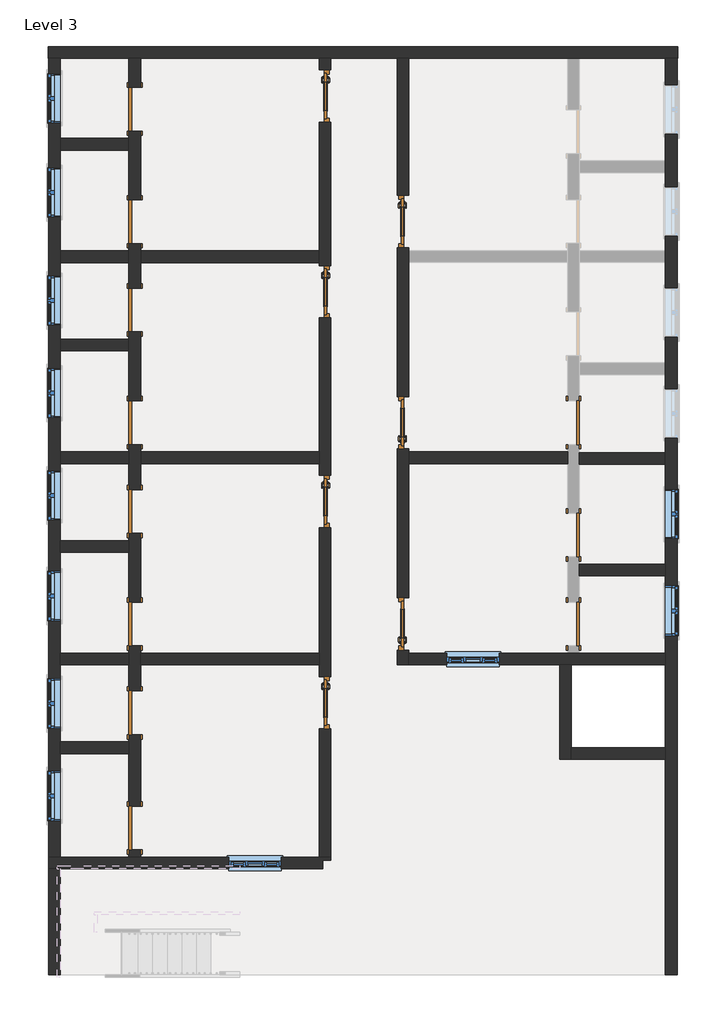
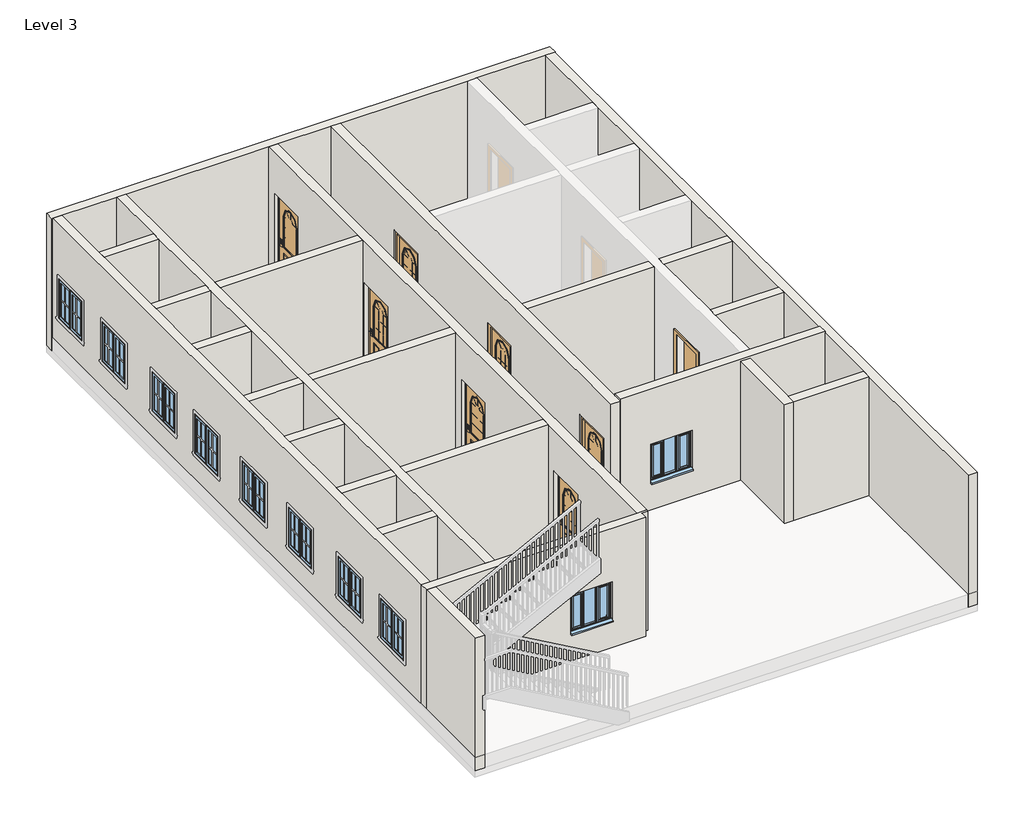
# One storey, part 1 of 4: 24 walls, 18 doors, 12 windows.
"""IFC4 building model written with IfcOpenShell, lengths in millimetres."""

from ifc_helpers import new_model, si_unit, frame, origin, place, context, project, spatial, polyline, outline, extrude, faceted_brep, transform, mapped, element, save
from components import doors_extsgl_w_glazing_bars_arched_910x2110mm_1ab485ba, doors_extsgl_w_glazing_bars_arched_910x2110mm_97dcda8a, door_fadea3f2, door_53b1b562, window_c29befe5, windows_tpl_plain_910x910mm_84e79c20

model = new_model("IFC4")

# Units and contexts
model_context = context("Model", 3, world=origin())
ifc_project = project(units=[si_unit("LENGTHUNIT", "METRE", prefix="MILLI")], contexts=[model_context])

# Site, building, storey
site = spatial("IfcSite", under=ifc_project)
building = spatial("IfcBuilding", under=site)
storey = spatial("IfcBuildingStorey", under=building, Name="Level 3", Elevation=6096.0)

# Doors
placement = place(None, origin())
doors_extsgl_w_glazing_bars_arched_910x2110mm_shape = doors_extsgl_w_glazing_bars_arched_910x2110mm_1ab485ba(model_context)
element("IfcDoor", 1, ObjectType="Doors_ExtSgl_w-Glazing_Bars_Arched : 910x2110mm", at=placement, inside=storey, context=model_context, shape_type="MappedRepresentation", body=[
    mapped(doors_extsgl_w_glazing_bars_arched_910x2110mm_shape, transform((-1635.1108866, 7135.2399728, 6096.0), x_axis=(0.0, -1.0, 0.0), y_axis=(1.0, 0.0, 0.0), z_axis=(0.0, 0.0, 1.0))),
])
element("IfcDoor", 2, ObjectType="Doors_ExtSgl_w-Glazing_Bars_Arched : 910x2110mm", at=placement, inside=storey, context=model_context, shape_type="MappedRepresentation", body=[
    mapped(doors_extsgl_w_glazing_bars_arched_910x2110mm_shape, transform((-1635.1108866, 3727.1935874, 6096.0), x_axis=(0.0, -1.0, 0.0), y_axis=(1.0, 0.0, 0.0), z_axis=(0.0, 0.0, 1.0))),
])
element("IfcDoor", 3, ObjectType="Doors_ExtSgl_w-Glazing_Bars_Arched : 910x2110mm", at=placement, inside=storey, context=model_context, shape_type="MappedRepresentation", body=[
    mapped(doors_extsgl_w_glazing_bars_arched_910x2110mm_shape, transform((-1635.1108866, 74.0399728, 6096.0), x_axis=(0.0, -1.0, 0.0), y_axis=(1.0, 0.0, 0.0), z_axis=(0.0, 0.0, 1.0))),
])
element("IfcDoor", 4, ObjectType="Doors_ExtSgl_w-Glazing_Bars_Arched : 910x2110mm", at=placement, inside=storey, context=model_context, shape_type="MappedRepresentation", body=[
    mapped(doors_extsgl_w_glazing_bars_arched_910x2110mm_shape, transform((-1635.1108866, -3431.1600272, 6096.0), x_axis=(0.0, -1.0, 0.0), y_axis=(1.0, 0.0, 0.0), z_axis=(0.0, 0.0, 1.0))),
])
element("IfcDoor", 5, ObjectType="Doors_ExtSgl_w-Glazing_Bars_Arched : 910x2110mm", at=placement, inside=storey, context=model_context, shape_type="MappedRepresentation", body=[
    mapped(doors_extsgl_w_glazing_bars_arched_910x2110mm_shape, transform((-276.2108866, -2059.5600272, 6096.0), x_axis=(0.0, 1.0, 0.0), y_axis=(-1.0, 0.0, 0.0), z_axis=(0.0, 0.0, 1.0))),
])
element("IfcDoor", 6, ObjectType="Doors_ExtSgl_w-Glazing_Bars_Arched : 910x2110mm", at=placement, inside=storey, context=model_context, shape_type="MappedRepresentation", body=[
    mapped(doors_extsgl_w_glazing_bars_arched_910x2110mm_shape, transform((-276.2108866, 1445.6399728, 6096.0), x_axis=(0.0, 1.0, 0.0), y_axis=(-1.0, 0.0, 0.0), z_axis=(0.0, 0.0, 1.0))),
])
doors_extsgl_w_glazing_bars_arched_910x2110mm_2_shape = doors_extsgl_w_glazing_bars_arched_910x2110mm_97dcda8a(model_context)
element("IfcDoor", 7, ObjectType="Doors_ExtSgl_w-Glazing_Bars_Arched : 910x2110mm", at=placement, inside=storey, context=model_context, shape_type="MappedRepresentation", body=[
    mapped(doors_extsgl_w_glazing_bars_arched_910x2110mm_2_shape, transform((-276.2108866, 4950.8399728, 6096.0), x_axis=(0.0, -1.0, 0.0), y_axis=(1.0, 0.0, 0.0), z_axis=(0.0, 0.0, 1.0))),
])
door_shape = door_fadea3f2(model_context)
element("IfcDoor", 8, ObjectType="Single-Flush : 30\" x 80\"", at=placement, inside=storey, context=model_context, shape_type="MappedRepresentation", body=[
    mapped(door_shape, transform((2695.5891134, -510.1600272, 6096.0), x_axis=(0.0, -1.0, 0.0), y_axis=(1.0, 0.0, 0.0), z_axis=(0.0, 0.0, 1.0))),
])
element("IfcDoor", 9, ObjectType="Single-Flush : 30\" x 80\"", at=placement, inside=storey, context=model_context, shape_type="MappedRepresentation", body=[
    mapped(door_shape, transform((2695.5891134, -2059.5600272, 6096.0), x_axis=(0.0, -1.0, 0.0), y_axis=(1.0, 0.0, 0.0), z_axis=(0.0, 0.0, 1.0))),
])
door_2_shape = door_53b1b562(model_context)
element("IfcDoor", 10, ObjectType="Single-Flush : 30\" x 80\"", at=placement, inside=storey, context=model_context, shape_type="MappedRepresentation", body=[
    mapped(door_2_shape, transform((-4949.8108866, 6906.6399728, 6096.0), x_axis=(0.0, -1.0, 0.0), y_axis=(1.0, 0.0, 0.0), z_axis=(0.0, 0.0, 1.0))),
])
element("IfcDoor", 11, ObjectType="Single-Flush : 30\" x 80\"", at=placement, inside=storey, context=model_context, shape_type="MappedRepresentation", body=[
    mapped(door_2_shape, transform((-4949.8108866, 4946.3935874, 6096.0), x_axis=(0.0, -1.0, 0.0), y_axis=(1.0, 0.0, 0.0), z_axis=(0.0, 0.0, 1.0))),
])
element("IfcDoor", 12, ObjectType="Single-Flush : 30\" x 80\"", at=placement, inside=storey, context=model_context, shape_type="MappedRepresentation", body=[
    mapped(door_2_shape, transform((-4949.8108866, 3407.538843, 6096.0), x_axis=(0.0, -1.0, 0.0), y_axis=(1.0, 0.0, 0.0), z_axis=(0.0, 0.0, 1.0))),
])
element("IfcDoor", 13, ObjectType="Single-Flush : 30\" x 80\"", at=placement, inside=storey, context=model_context, shape_type="MappedRepresentation", body=[
    mapped(door_2_shape, transform((-4949.8108866, 1445.6399728, 6096.0), x_axis=(0.0, -1.0, 0.0), y_axis=(1.0, 0.0, 0.0), z_axis=(0.0, 0.0, 1.0))),
])
element("IfcDoor", 14, ObjectType="Single-Flush : 30\" x 80\"", at=placement, inside=storey, context=model_context, shape_type="MappedRepresentation", body=[
    mapped(door_2_shape, transform((-4949.8108866, -103.7600272, 6096.0), x_axis=(0.0, -1.0, 0.0), y_axis=(1.0, 0.0, 0.0), z_axis=(0.0, 0.0, 1.0))),
])
element("IfcDoor", 15, ObjectType="Single-Flush : 30\" x 80\"", at=placement, inside=storey, context=model_context, shape_type="MappedRepresentation", body=[
    mapped(door_2_shape, transform((-4949.8108866, -2059.5600272, 6096.0), x_axis=(0.0, -1.0, 0.0), y_axis=(1.0, 0.0, 0.0), z_axis=(0.0, 0.0, 1.0))),
])
element("IfcDoor", 16, ObjectType="Single-Flush : 30\" x 80\"", at=placement, inside=storey, context=model_context, shape_type="MappedRepresentation", body=[
    mapped(door_2_shape, transform((-4949.8108866, -3608.9600272, 6096.0), x_axis=(0.0, -1.0, 0.0), y_axis=(1.0, 0.0, 0.0), z_axis=(0.0, 0.0, 1.0))),
])
element("IfcDoor", 17, ObjectType="Single-Flush : 30\" x 80\"", at=placement, inside=storey, context=model_context, shape_type="MappedRepresentation", body=[
    mapped(door_2_shape, transform((-4949.8108866, -5615.5600272, 6096.0), x_axis=(0.0, -1.0, 0.0), y_axis=(1.0, 0.0, 0.0), z_axis=(0.0, 0.0, 1.0))),
])
element("IfcDoor", 18, ObjectType="Single-Flush : 30\" x 80\"", at=placement, inside=storey, context=model_context, shape_type="MappedRepresentation", body=[
    mapped(door_2_shape, transform((2695.5891134, 1445.6399728, 6096.0), x_axis=(0.0, 1.0, 0.0), y_axis=(-1.0, 0.0, 0.0), z_axis=(0.0, 0.0, 1.0))),
])

# Walls
element("IfcWall", 19, ObjectType="4.5\" p", at=placement, inside=storey, context=model_context, shape_type="Brep", body=[
    faceted_brep([(-5051.4108866, -5996.5600272, 8128.0), (-5051.4108866, -5996.5600272, 6096.0), (-5051.4108866, -6123.5600272, 6096.0), (-5051.4108866, -6123.5600272, 9144.0), (-5051.4108866, -4320.1600272, 9144.0), (-5051.4108866, -4116.9600272, 9144.0), (-5051.4108866, -2770.7600272, 9144.0), (-5051.4108866, -2567.5600272, 9144.0), (-5051.4108866, -814.9600272, 9144.0), (-5051.4108866, -611.7600272, 9144.0), (-5051.4108866, 734.4399728, 9144.0), (-5051.4108866, 937.6399728, 9144.0), (-5051.4108866, 2696.338843, 9144.0), (-5051.4108866, 2899.538843, 9144.0), (-5051.4108866, 4235.1935874, 9144.0), (-5051.4108866, 4438.3935874, 9144.0), (-5051.4108866, 6195.4399728, 9144.0), (-5051.4108866, 6398.6399728, 9144.0), (-5051.4108866, 7795.6399728, 9144.0), (-5051.4108866, 7795.6399728, 6096.0), (-5051.4108866, 7287.6399728, 6096.0), (-5051.4108866, 7287.6399728, 8128.0), (-5051.4108866, 6525.6399728, 8128.0), (-5051.4108866, 6525.6399728, 6096.0), (-5051.4108866, 6398.6399728, 6096.0), (-5051.4108866, 6195.4399728, 6096.0), (-5051.4108866, 5327.3935874, 6096.0), (-5051.4108866, 5327.3935874, 8128.0), (-5051.4108866, 4565.3935874, 8128.0), (-5051.4108866, 4565.3935874, 6096.0), (-5051.4108866, 4438.3935874, 6096.0), (-5051.4108866, 4235.1935874, 6096.0), (-5051.4108866, 3788.538843, 6096.0), (-5051.4108866, 3788.538843, 8128.0), (-5051.4108866, 3026.538843, 8128.0), (-5051.4108866, 3026.538843, 6096.0), (-5051.4108866, 2899.538843, 6096.0), (-5051.4108866, 2696.338843, 6096.0), (-5051.4108866, 1826.6399728, 6096.0), (-5051.4108866, 1826.6399728, 8128.0), (-5051.4108866, 1064.6399728, 8128.0), (-5051.4108866, 1064.6399728, 6096.0), (-5051.4108866, 937.6399728, 6096.0), (-5051.4108866, 734.4399728, 6096.0), (-5051.4108866, 277.2399728, 6096.0), (-5051.4108866, 277.2399728, 8128.0), (-5051.4108866, -484.7600272, 8128.0), (-5051.4108866, -484.7600272, 6096.0), (-5051.4108866, -611.7600272, 6096.0), (-5051.4108866, -814.9600272, 6096.0), (-5051.4108866, -1678.5600272, 6096.0), (-5051.4108866, -1678.5600272, 8128.0), (-5051.4108866, -2440.5600272, 8128.0), (-5051.4108866, -2440.5600272, 6096.0), (-5051.4108866, -2567.5600272, 6096.0), (-5051.4108866, -2770.7600272, 6096.0), (-5051.4108866, -3227.9600272, 6096.0), (-5051.4108866, -3227.9600272, 8128.0), (-5051.4108866, -3989.9600272, 8128.0), (-5051.4108866, -3989.9600272, 6096.0), (-5051.4108866, -4116.9600272, 6096.0), (-5051.4108866, -4320.1600272, 6096.0), (-5051.4108866, -5234.5600272, 6096.0), (-5051.4108866, -5234.5600272, 8128.0), (-4848.2108866, -6123.5600272, 6096.0), (-4848.2108866, -5996.5600272, 6096.0), (-4848.2108866, -5996.5600272, 8128.0), (-4848.2108866, -5234.5600272, 8128.0), (-4848.2108866, -5234.5600272, 6096.0), (-4848.2108866, -3989.9600272, 6096.0), (-4848.2108866, -3989.9600272, 8128.0), (-4848.2108866, -3227.9600272, 8128.0), (-4848.2108866, -3227.9600272, 6096.0), (-4848.2108866, -2770.7600272, 6096.0), (-4848.2108866, -2567.5600272, 6096.0), (-4848.2108866, -2440.5600272, 6096.0), (-4848.2108866, -2440.5600272, 8128.0), (-4848.2108866, -1678.5600272, 8128.0), (-4848.2108866, -1678.5600272, 6096.0), (-4848.2108866, -484.7600272, 6096.0), (-4848.2108866, -484.7600272, 8128.0), (-4848.2108866, 277.2399728, 8128.0), (-4848.2108866, 277.2399728, 6096.0), (-4848.2108866, 734.4399728, 6096.0), (-4848.2108866, 937.6399728, 6096.0), (-4848.2108866, 1064.6399728, 6096.0), (-4848.2108866, 1064.6399728, 8128.0), (-4848.2108866, 1826.6399728, 8128.0), (-4848.2108866, 1826.6399728, 6096.0), (-4848.2108866, 3026.538843, 6096.0), (-4848.2108866, 3026.538843, 8128.0), (-4848.2108866, 3788.538843, 8128.0), (-4848.2108866, 3788.538843, 6096.0), (-4848.2108866, 4235.1935874, 6096.0), (-4848.2108866, 4438.3935874, 6096.0), (-4848.2108866, 4565.3935874, 6096.0), (-4848.2108866, 4565.3935874, 8128.0), (-4848.2108866, 5327.3935874, 8128.0), (-4848.2108866, 5327.3935874, 6096.0), (-4848.2108866, 6525.6399728, 6096.0), (-4848.2108866, 6525.6399728, 8128.0), (-4848.2108866, 7287.6399728, 8128.0), (-4848.2108866, 7287.6399728, 6096.0), (-4848.2108866, 7795.6399728, 6096.0), (-4848.2108866, 7795.6399728, 9144.0), (-4848.2108866, 4438.3935874, 9144.0), (-4848.2108866, 4235.1935874, 9144.0), (-4848.2108866, 937.6399728, 9144.0), (-4848.2108866, 734.4399728, 9144.0), (-4848.2108866, -2567.5600272, 9144.0), (-4848.2108866, -2770.7600272, 9144.0), (-4848.2108866, -6123.5600272, 9144.0)], [[[0, 1, 2, 3, 4, 5, 6, 7, 8, 9, 10, 11, 12, 13, 14, 15, 16, 17, 18, 19, 20, 21, 22, 23, 24, 25, 26, 27, 28, 29, 30, 31, 32, 33, 34, 35, 36, 37, 38, 39, 40, 41, 42, 43, 44, 45, 46, 47, 48, 49, 50, 51, 52, 53, 54, 55, 56, 57, 58, 59, 60, 61, 62, 63]], [[64, 65, 66, 67, 68, 69, 70, 71, 72, 73, 74, 75, 76, 77, 78, 79, 80, 81, 82, 83, 84, 85, 86, 87, 88, 89, 90, 91, 92, 93, 94, 95, 96, 97, 98, 99, 100, 101, 102, 103, 104, 105, 106, 107, 108, 109, 110, 111]], [[20, 19, 103, 102]], [[26, 25, 24, 23, 99, 98]], [[32, 31, 30, 29, 95, 94, 93, 92]], [[38, 37, 36, 35, 89, 88]], [[44, 43, 42, 41, 85, 84, 83, 82]], [[50, 49, 48, 47, 79, 78]], [[56, 55, 54, 53, 75, 74, 73, 72]], [[2, 1, 65, 64]], [[62, 61, 60, 59, 69, 68]], [[18, 17, 16, 15, 14, 13, 12, 11, 10, 9, 8, 7, 6, 5, 4, 3, 111, 110, 109, 108, 107, 106, 105, 104]], [[19, 18, 104, 103]], [[3, 2, 64, 111]], [[100, 99, 23, 22]], [[101, 100, 22, 21]], [[102, 101, 21, 20]], [[96, 95, 29, 28]], [[97, 96, 28, 27]], [[98, 97, 27, 26]], [[90, 89, 35, 34]], [[91, 90, 34, 33]], [[92, 91, 33, 32]], [[86, 85, 41, 40]], [[87, 86, 40, 39]], [[88, 87, 39, 38]], [[80, 79, 47, 46]], [[81, 80, 46, 45]], [[82, 81, 45, 44]], [[76, 75, 53, 52]], [[77, 76, 52, 51]], [[78, 77, 51, 50]], [[70, 69, 59, 58]], [[71, 70, 58, 57]], [[72, 71, 57, 56]], [[66, 65, 1, 0]], [[67, 66, 0, 63]], [[68, 67, 63, 62]]]),
])
element("IfcWall", 20, ObjectType="4.5\" p", at=placement, inside=storey, context=model_context, shape_type="SweptSolid", body=[
    extrude(outline(polyline([(-5051.4108866, 6195.4399728), (-6245.2108866, 6195.4399728), (-6245.2108866, 6398.6399728), (-5051.4108866, 6398.6399728), (-5051.4108866, 6195.4399728)])), frame((0.0, 0.0, 6096.0), z_axis=(0.0, 0.0, 1.0), x_axis=(1.0, 0.0, 0.0)), (0.0, 0.0, 1.0), 3048.0),
])
element("IfcWall", 21, ObjectType="4.5\" p", at=placement, inside=storey, context=model_context, shape_type="SweptSolid", body=[
    extrude(outline(polyline([(-5051.4108866, 4235.1935874), (-6245.2108866, 4235.1935874), (-6245.2108866, 4438.3935874), (-5051.4108866, 4438.3935874), (-5051.4108866, 4235.1935874)])), frame((0.0, 0.0, 6096.0), z_axis=(0.0, 0.0, 1.0), x_axis=(1.0, 0.0, 0.0)), (0.0, 0.0, 1.0), 3048.0),
])
element("IfcWall", 22, ObjectType="4.5\" p", at=placement, inside=storey, context=model_context, shape_type="SweptSolid", body=[
    extrude(outline(polyline([(-5051.4108866, 2696.338843), (-6245.2108866, 2696.338843), (-6245.2108866, 2899.538843), (-5051.4108866, 2899.538843), (-5051.4108866, 2696.338843)])), frame((0.0, 0.0, 6096.0), z_axis=(0.0, 0.0, 1.0), x_axis=(1.0, 0.0, 0.0)), (0.0, 0.0, 1.0), 3048.0),
])
element("IfcWall", 23, ObjectType="4.5\" p", at=placement, inside=storey, context=model_context, shape_type="SweptSolid", body=[
    extrude(outline(polyline([(-5051.4108866, 734.4399728), (-6245.2108866, 734.4399728), (-6245.2108866, 937.6399728), (-5051.4108866, 937.6399728), (-5051.4108866, 734.4399728)])), frame((0.0, 0.0, 6096.0), z_axis=(0.0, 0.0, 1.0), x_axis=(1.0, 0.0, 0.0)), (0.0, 0.0, 1.0), 3048.0),
])
element("IfcWall", 24, ObjectType="4.5\" p", at=placement, inside=storey, context=model_context, shape_type="SweptSolid", body=[
    extrude(outline(polyline([(-5051.4108866, -814.9600272), (-6245.2108866, -814.9600272), (-6245.2108866, -611.7600272), (-5051.4108866, -611.7600272), (-5051.4108866, -814.9600272)])), frame((0.0, 0.0, 6096.0), z_axis=(0.0, 0.0, 1.0), x_axis=(1.0, 0.0, 0.0)), (0.0, 0.0, 1.0), 3048.0),
])
element("IfcWall", 25, ObjectType="4.5\" p", at=placement, inside=storey, context=model_context, shape_type="SweptSolid", body=[
    extrude(outline(polyline([(-5051.4108866, -2770.7600272), (-6245.2108866, -2770.7600272), (-6245.2108866, -2567.5600272), (-5051.4108866, -2567.5600272), (-5051.4108866, -2770.7600272)])), frame((0.0, 0.0, 6096.0), z_axis=(0.0, 0.0, 1.0), x_axis=(1.0, 0.0, 0.0)), (0.0, 0.0, 1.0), 3048.0),
])
element("IfcWall", 26, ObjectType="4.5\" p", at=placement, inside=storey, context=model_context, shape_type="SweptSolid", body=[
    extrude(outline(polyline([(-5051.4108866, -4320.1600272), (-6245.2108866, -4320.1600272), (-6245.2108866, -4116.9600272), (-5051.4108866, -4116.9600272), (-5051.4108866, -4320.1600272)])), frame((0.0, 0.0, 6096.0), z_axis=(0.0, 0.0, 1.0), x_axis=(1.0, 0.0, 0.0)), (0.0, 0.0, 1.0), 3048.0),
])
element("IfcWall", 27, ObjectType="4.5\" p", at=placement, inside=storey, context=model_context, shape_type="Brep", body=[
    faceted_brep([(-1736.7108866, -3886.1600272, 8206.0), (-1736.7108866, -3886.1600272, 6096.0), (-1736.7108866, -6123.5600272, 6096.0), (-1736.7108866, -6123.5600272, 9144.0), (-1736.7108866, -2770.7600272, 9144.0), (-1736.7108866, -2567.5600272, 9144.0), (-1736.7108866, 734.4399728, 9144.0), (-1736.7108866, 937.6399728, 9144.0), (-1736.7108866, 4235.1935874, 9144.0), (-1736.7108866, 4438.3935874, 9144.0), (-1736.7108866, 7795.6399728, 9144.0), (-1736.7108866, 7795.6399728, 6096.0), (-1736.7108866, 7590.2399728, 6096.0), (-1736.7108866, 7590.2399728, 8206.0), (-1736.7108866, 6680.2399728, 8206.0), (-1736.7108866, 6680.2399728, 6096.0), (-1736.7108866, 4438.3935874, 6096.0), (-1736.7108866, 4235.1935874, 6096.0), (-1736.7108866, 4182.1935874, 6096.0), (-1736.7108866, 4182.1935874, 8206.0), (-1736.7108866, 3272.1935874, 8206.0), (-1736.7108866, 3272.1935874, 6096.0), (-1736.7108866, 937.6399728, 6096.0), (-1736.7108866, 734.4399728, 6096.0), (-1736.7108866, 529.0399728, 6096.0), (-1736.7108866, 529.0399728, 8206.0), (-1736.7108866, -380.9600272, 8206.0), (-1736.7108866, -380.9600272, 6096.0), (-1736.7108866, -2567.5600272, 6096.0), (-1736.7108866, -2770.7600272, 6096.0), (-1736.7108866, -2976.1600272, 6096.0), (-1736.7108866, -2976.1600272, 8206.0), (-1533.5108866, -6123.5600272, 6096.0), (-1533.5108866, -3886.1600272, 6096.0), (-1533.5108866, -3886.1600272, 8206.0), (-1533.5108866, -2976.1600272, 8206.0), (-1533.5108866, -2976.1600272, 6096.0), (-1533.5108866, -380.9600272, 6096.0), (-1533.5108866, -380.9600272, 8206.0), (-1533.5108866, 529.0399728, 8206.0), (-1533.5108866, 529.0399728, 6096.0), (-1533.5108866, 3272.1935874, 6096.0), (-1533.5108866, 3272.1935874, 8206.0), (-1533.5108866, 4182.1935874, 8206.0), (-1533.5108866, 4182.1935874, 6096.0), (-1533.5108866, 6680.2399728, 6096.0), (-1533.5108866, 6680.2399728, 8206.0), (-1533.5108866, 7590.2399728, 8206.0), (-1533.5108866, 7590.2399728, 6096.0), (-1533.5108866, 7795.6399728, 6096.0), (-1533.5108866, 7795.6399728, 9144.0), (-1533.5108866, -6123.5600272, 9144.0)], [[[0, 1, 2, 3, 4, 5, 6, 7, 8, 9, 10, 11, 12, 13, 14, 15, 16, 17, 18, 19, 20, 21, 22, 23, 24, 25, 26, 27, 28, 29, 30, 31]], [[32, 33, 34, 35, 36, 37, 38, 39, 40, 41, 42, 43, 44, 45, 46, 47, 48, 49, 50, 51]], [[12, 11, 49, 48]], [[18, 17, 16, 15, 45, 44]], [[24, 23, 22, 21, 41, 40]], [[2, 1, 33, 32]], [[30, 29, 28, 27, 37, 36]], [[10, 9, 8, 7, 6, 5, 4, 3, 51, 50]], [[3, 2, 32, 51]], [[11, 10, 50, 49]], [[48, 47, 13, 12]], [[46, 45, 15, 14]], [[47, 46, 14, 13]], [[44, 43, 19, 18]], [[42, 41, 21, 20]], [[43, 42, 20, 19]], [[40, 39, 25, 24]], [[38, 37, 27, 26]], [[39, 38, 26, 25]], [[36, 35, 31, 30]], [[34, 33, 1, 0]], [[35, 34, 0, 31]]]),
])
element("IfcWall", 28, ObjectType="4.5\" p", at=placement, inside=storey, context=model_context, shape_type="SweptSolid", body=[
    extrude(outline(polyline([(-1736.7108866, 4235.1935874), (-4848.2108866, 4235.1935874), (-4848.2108866, 4438.3935874), (-1736.7108866, 4438.3935874), (-1736.7108866, 4235.1935874)])), frame((0.0, 0.0, 6096.0), z_axis=(0.0, 0.0, 1.0), x_axis=(1.0, 0.0, 0.0)), (0.0, 0.0, 1.0), 3048.0),
])
element("IfcWall", 29, ObjectType="4.5\" p", at=placement, inside=storey, context=model_context, shape_type="SweptSolid", body=[
    extrude(outline(polyline([(-1736.7108866, 734.4399728), (-4848.2108866, 734.4399728), (-4848.2108866, 937.6399728), (-1736.7108866, 937.6399728), (-1736.7108866, 734.4399728)])), frame((0.0, 0.0, 6096.0), z_axis=(0.0, 0.0, 1.0), x_axis=(1.0, 0.0, 0.0)), (0.0, 0.0, 1.0), 3048.0),
])
element("IfcWall", 30, ObjectType="4.5\" p", at=placement, inside=storey, context=model_context, shape_type="SweptSolid", body=[
    extrude(outline(polyline([(-1736.7108866, -2770.7600272), (-4848.2108866, -2770.7600272), (-4848.2108866, -2567.5600272), (-1736.7108866, -2567.5600272), (-1736.7108866, -2770.7600272)])), frame((0.0, 0.0, 6096.0), z_axis=(0.0, 0.0, 1.0), x_axis=(1.0, 0.0, 0.0)), (0.0, 0.0, 1.0), 3048.0),
])
element("IfcWall", 31, ObjectType="4.5\" p", at=placement, inside=storey, context=model_context, shape_type="Brep", body=[
    faceted_brep([(-377.8108866, 4495.8399728, 8206.0), (-377.8108866, 4495.8399728, 6096.0), (-377.8108866, 1900.6399728, 6096.0), (-377.8108866, 1900.6399728, 8206.0), (-377.8108866, 990.6399728, 8206.0), (-377.8108866, 990.6399728, 6096.0), (-377.8108866, -1604.5600272, 6096.0), (-377.8108866, -1604.5600272, 8206.0), (-377.8108866, -2514.5600272, 8206.0), (-377.8108866, -2514.5600272, 6096.0), (-377.8108866, -2770.7600272, 6096.0), (-377.8108866, -2770.7600272, 9144.0), (-377.8108866, 7795.6399728, 9144.0), (-377.8108866, 7795.6399728, 6096.0), (-377.8108866, 5405.8399728, 6096.0), (-377.8108866, 5405.8399728, 8206.0), (-174.6108866, 1900.6399728, 6096.0), (-174.6108866, 4239.6399728, 6096.0), (-174.6108866, 4442.8399728, 6096.0), (-174.6108866, 4495.8399728, 6096.0), (-174.6108866, 4495.8399728, 8206.0), (-174.6108866, 5405.8399728, 8206.0), (-174.6108866, 5405.8399728, 6096.0), (-174.6108866, 7795.6399728, 6096.0), (-174.6108866, 7795.6399728, 9144.0), (-174.6108866, 4442.8399728, 9144.0), (-174.6108866, 4239.6399728, 9144.0), (-174.6108866, 937.6399728, 9144.0), (-174.6108866, 734.4399728, 9144.0), (-174.6108866, -2770.7600272, 9144.0), (-174.6108866, -2770.7600272, 6096.0), (-174.6108866, -2567.5600272, 6096.0), (-174.6108866, -2514.5600272, 6096.0), (-174.6108866, -2514.5600272, 8206.0), (-174.6108866, -1604.5600272, 8206.0), (-174.6108866, -1604.5600272, 6096.0), (-174.6108866, 734.4399728, 6096.0), (-174.6108866, 937.6399728, 6096.0), (-174.6108866, 990.6399728, 6096.0), (-174.6108866, 990.6399728, 8206.0), (-174.6108866, 1900.6399728, 8206.0)], [[[0, 1, 2, 3, 4, 5, 6, 7, 8, 9, 10, 11, 12, 13, 14, 15]], [[16, 17, 18, 19, 20, 21, 22, 23, 24, 25, 26, 27, 28, 29, 30, 31, 32, 33, 34, 35, 36, 37, 38, 39, 40]], [[32, 31, 30, 10, 9]], [[38, 37, 36, 35, 6, 5]], [[14, 13, 23, 22]], [[2, 1, 19, 18, 17, 16]], [[12, 11, 29, 28, 27, 26, 25, 24]], [[13, 12, 24, 23]], [[11, 10, 30, 29]], [[9, 8, 33, 32]], [[7, 6, 35, 34]], [[8, 7, 34, 33]], [[5, 4, 39, 38]], [[3, 2, 16, 40]], [[4, 3, 40, 39]], [[22, 21, 15, 14]], [[20, 19, 1, 0]], [[21, 20, 0, 15]]]),
])
element("IfcWall", 32, ObjectType="4.5\" p", at=placement, inside=storey, context=model_context, shape_type="Brep", body=[
    faceted_brep([(-174.6108866, -2770.7600272, 6096.0), (2454.2891134, -2770.7600272, 6096.0), (2657.4891134, -2770.7600272, 6096.0), (4295.7891134, -2770.7600272, 6096.0), (4295.7891134, -2770.7600272, 9184.1226014), (-174.6108866, -2770.7600272, 9184.1226014), (-174.6108866, -2770.7600272, 9144.0), (1397.9891134, -2770.7600272, 7920.4), (1397.9891134, -2770.7600272, 7010.4), (487.9891134, -2770.7600272, 7010.4), (487.9891134, -2770.7600272, 7920.4), (-174.6108866, -2567.5600272, 6096.0), (-174.6108866, -2567.5600272, 9184.1226014), (4295.7891134, -2567.5600272, 9184.1226014), (4295.7891134, -2567.5600272, 6096.0), (2797.1891134, -2567.5600272, 6096.0), (2593.9891134, -2567.5600272, 6096.0), (1397.9891134, -2567.5600272, 7920.4), (487.9891134, -2567.5600272, 7920.4), (487.9891134, -2567.5600272, 7010.4), (1397.9891134, -2567.5600272, 7010.4)], [[[0, 1, 2, 3, 4, 5, 6], [7, 8, 9, 10]], [[11, 12, 13, 14, 15, 16], [17, 18, 19, 20]], [[3, 2, 1, 0, 11, 16, 15, 14]], [[5, 4, 13, 12]], [[0, 6, 5, 12, 11]], [[4, 3, 14, 13]], [[8, 7, 17, 20]], [[9, 8, 20, 19]], [[10, 9, 19, 18]], [[7, 10, 18, 17]]]),
])
element("IfcWall", 33, ObjectType="4.5\" p", at=placement, inside=storey, context=model_context, shape_type="Brep", body=[
    faceted_brep([(2454.2891134, -2770.7600272, 6096.0), (2454.2891134, -4421.7600272, 6096.0), (2454.2891134, -4421.7600272, 9144.0), (2454.2891134, -2770.7600272, 9144.0), (2657.4891134, -2770.7600272, 6096.0), (2657.4891134, -2770.7600272, 9144.0), (2657.4891134, -4218.5600272, 9144.0), (2657.4891134, -4421.7600272, 9144.0), (2657.4891134, -4421.7600272, 6096.0), (2657.4891134, -4218.5600272, 6096.0)], [[[0, 1, 2, 3]], [[4, 5, 6, 7, 8, 9]], [[1, 0, 4, 9, 8]], [[3, 2, 7, 6, 5]], [[0, 3, 5, 4]], [[2, 1, 8, 7]]]),
])
element("IfcWall", 34, ObjectType="4.5\" p", at=placement, inside=storey, context=model_context, shape_type="SweptSolid", body=[
    extrude(outline(polyline([(2657.4891134, -4218.5600272), (4295.7891134, -4218.5600272), (4295.7891134, -4421.7600272), (2657.4891134, -4421.7600272), (2657.4891134, -4218.5600272)])), frame((0.0, 0.0, 6096.0), z_axis=(0.0, 0.0, 1.0), x_axis=(1.0, 0.0, 0.0)), (0.0, 0.0, 1.0), 3048.0),
])
element("IfcWall", 35, ObjectType="4.5\" p", at=placement, inside=storey, context=model_context, shape_type="SweptSolid", body=[
    extrude(outline(polyline([(4295.7891134, 721.7399728), (2797.1891134, 721.7399728), (2797.1891134, 924.9399728), (4295.7891134, 924.9399728), (4295.7891134, 721.7399728)])), frame((0.0, 0.0, 6096.0), z_axis=(0.0, 0.0, 1.0), x_axis=(1.0, 0.0, 0.0)), (0.0, 0.0, 1.0), 3048.0),
])
element("IfcWall", 36, ObjectType="4.5\" p", at=placement, inside=storey, context=model_context, shape_type="SweptSolid", body=[
    extrude(outline(polyline([(4295.7891134, -1221.3600272), (2797.1891134, -1221.3600272), (2797.1891134, -1018.1600272), (4295.7891134, -1018.1600272), (4295.7891134, -1221.3600272)])), frame((0.0, 0.0, 6096.0), z_axis=(0.0, 0.0, 1.0), x_axis=(1.0, 0.0, 0.0)), (0.0, 0.0, 1.0), 3048.0),
])
element("IfcWall", 37, ObjectType="4.5\" p", at=placement, inside=storey, context=model_context, shape_type="SweptSolid", body=[
    extrude(outline(polyline([(2593.9891134, 734.4399728), (-174.6108866, 734.4399728), (-174.6108866, 937.6399728), (2593.9891134, 937.6399728), (2593.9891134, 734.4399728)])), frame((0.0, 0.0, 6096.0), z_axis=(0.0, 0.0, 1.0), x_axis=(1.0, 0.0, 0.0)), (0.0, 0.0, 1.0), 3048.0),
])
element("IfcWall", 38, ObjectType="4.5\" p", at=placement, inside=storey, context=model_context, shape_type="SweptSolid", body=[
    extrude(outline(polyline([(-6448.4108866, -8168.2600272), (-6448.4108866, -6326.7600272), (-6245.2108866, -6326.7600272), (-6245.2108866, -8168.2600272), (-6448.4108866, -8168.2600272)])), frame((0.0, 0.0, 6096.0), z_axis=(0.0, 0.0, 1.0), x_axis=(1.0, 0.0, 0.0)), (0.0, 0.0, 1.0), 3048.0),
])
element("IfcWall", 39, ObjectType="9\" w", at=placement, inside=storey, context=model_context, shape_type="Brep", body=[
    faceted_brep([(-6461.1108866, 7795.6399728, 6096.0), (-6448.4108866, 7795.6399728, 6096.0), (-6245.2108866, 7795.6399728, 6096.0), (-5051.4108866, 7795.6399728, 6096.0), (-4848.2108866, 7795.6399728, 6096.0), (-1736.7108866, 7795.6399728, 6096.0), (-1533.5108866, 7795.6399728, 6096.0), (-377.8108866, 7795.6399728, 6096.0), (-174.6108866, 7795.6399728, 6096.0), (2593.9891134, 7795.6399728, 6096.0), (2797.1891134, 7795.6399728, 6096.0), (4295.7891134, 7795.6399728, 6096.0), (4498.9891134, 7795.6399728, 6096.0), (4511.6891134, 7795.6399728, 6096.0), (4511.6891134, 7795.6399728, 9144.0), (4498.9891134, 7795.6399728, 9144.0), (4295.7891134, 7795.6399728, 9144.0), (2797.1891134, 7795.6399728, 9144.0), (2593.9891134, 7795.6399728, 9144.0), (-174.6108866, 7795.6399728, 9144.0), (-377.8108866, 7795.6399728, 9144.0), (-1533.5108866, 7795.6399728, 9144.0), (-1736.7108866, 7795.6399728, 9144.0), (-4848.2108866, 7795.6399728, 9144.0), (-5051.4108866, 7795.6399728, 9144.0), (-6245.2108866, 7795.6399728, 9144.0), (-6448.4108866, 7795.6399728, 9144.0), (-6461.1108866, 7795.6399728, 9144.0), (-6461.1108866, 7998.8399728, 6096.0), (-6461.1108866, 7998.8399728, 9144.0), (4511.6891134, 7998.8399728, 9144.0), (4511.6891134, 7998.8399728, 6096.0)], [[[0, 1, 2, 3, 4, 5, 6, 7, 8, 9, 10, 11, 12, 13, 14, 15, 16, 17, 18, 19, 20, 21, 22, 23, 24, 25, 26, 27]], [[28, 29, 30, 31]], [[13, 12, 11, 10, 9, 8, 7, 6, 5, 4, 3, 2, 1, 0, 28, 31]], [[14, 13, 31, 30]], [[27, 26, 25, 24, 23, 22, 21, 20, 19, 18, 17, 16, 15, 14, 30, 29]], [[0, 27, 29, 28]]]),
])
element("IfcWall", 40, ObjectType="9\" w", at=placement, inside=storey, context=model_context, shape_type="Brep", body=[
    faceted_brep([(-6448.4108866, -6326.7600272, 9144.0), (-6448.4108866, -6326.7600272, 6096.0), (-6245.2108866, -6326.7600272, 6096.0), (-1673.2108866, -6326.7600272, 6096.0), (-1673.2108866, -6326.7600272, 9144.0), (-6245.2108866, -6326.7600272, 9144.0), (-2399.3108866, -6326.7600272, 7920.4), (-2399.3108866, -6326.7600272, 7010.4), (-3309.3108866, -6326.7600272, 7010.4), (-3309.3108866, -6326.7600272, 7920.4), (-1533.5108866, -6123.5600272, 6096.0), (-1736.7108866, -6123.5600272, 6096.0), (-4848.2108866, -6123.5600272, 6096.0), (-5051.4108866, -6123.5600272, 6096.0), (-6245.2108866, -6123.5600272, 6096.0), (-6448.4108866, -6123.5600272, 6096.0), (-6448.4108866, -6123.5600272, 9144.0), (-6245.2108866, -6123.5600272, 9144.0), (-5051.4108866, -6123.5600272, 9144.0), (-4848.2108866, -6123.5600272, 9144.0), (-1736.7108866, -6123.5600272, 9144.0), (-1533.5108866, -6123.5600272, 9144.0), (-2399.3108866, -6123.5600272, 7010.4), (-2399.3108866, -6123.5600272, 7920.4), (-3309.3108866, -6123.5600272, 7920.4), (-3309.3108866, -6123.5600272, 7010.4), (-1533.5108866, -6174.3600272, 6096.0), (-1673.2108866, -6174.3600272, 6096.0), (-1673.2108866, -6174.3600272, 9144.0), (-1533.5108866, -6174.3600272, 9144.0)], [[[0, 1, 2, 3, 4, 5], [6, 7, 8, 9]], [[10, 11, 12, 13, 14, 15, 16, 17, 18, 19, 20, 21], [22, 23, 24, 25]], [[15, 14, 13, 12, 11, 10, 26, 27, 3, 2, 1]], [[21, 20, 19, 18, 17, 16, 0, 5, 4, 28, 29]], [[1, 0, 16, 15]], [[10, 21, 29, 26]], [[7, 6, 23, 22]], [[8, 7, 22, 25]], [[9, 8, 25, 24]], [[6, 9, 24, 23]], [[28, 27, 26, 29]], [[27, 28, 4, 3]]]),
])
element("IfcWall", 41, ObjectType="9\" w", at=placement, inside=storey, context=model_context, shape_type="Brep", body=[
    faceted_brep([(-6448.4108866, 7795.6399728, 6096.0), (-6448.4108866, -6123.5600272, 6096.0), (-6448.4108866, -6123.5600272, 9144.0), (-6448.4108866, 7795.6399728, 9144.0), (-6448.4108866, 7528.9399728, 7924.8), (-6448.4108866, 6665.3399728, 7924.8), (-6448.4108866, 6665.3399728, 7010.4), (-6448.4108866, 7528.9399728, 7010.4), (-6448.4108866, 5890.6399728, 7924.8), (-6448.4108866, 5027.0399728, 7924.8), (-6448.4108866, 5027.0399728, 7010.4), (-6448.4108866, 5890.6399728, 7010.4), (-6448.4108866, 4006.5935874, 7924.8), (-6448.4108866, 3142.9935874, 7924.8), (-6448.4108866, 3142.9935874, 7010.4), (-6448.4108866, 4006.5935874, 7010.4), (-6448.4108866, 2391.538843, 7924.8), (-6448.4108866, 1527.938843, 7924.8), (-6448.4108866, 1527.938843, 7010.4), (-6448.4108866, 2391.538843, 7010.4), (-6448.4108866, 607.4399728, 7924.8), (-6448.4108866, -256.1600272, 7924.8), (-6448.4108866, -256.1600272, 7010.4), (-6448.4108866, 607.4399728, 7010.4), (-6448.4108866, -1145.1600272, 7924.8), (-6448.4108866, -2008.7600272, 7924.8), (-6448.4108866, -2008.7600272, 7010.4), (-6448.4108866, -1145.1600272, 7010.4), (-6448.4108866, -3012.0600272, 7924.8), (-6448.4108866, -3875.6600272, 7924.8), (-6448.4108866, -3875.6600272, 7010.4), (-6448.4108866, -3012.0600272, 7010.4), (-6448.4108866, -4624.9600272, 7924.8), (-6448.4108866, -5488.5600272, 7924.8), (-6448.4108866, -5488.5600272, 7010.4), (-6448.4108866, -4624.9600272, 7010.4), (-6245.2108866, 7795.6399728, 6096.0), (-6245.2108866, 7795.6399728, 9144.0), (-6245.2108866, 6398.6399728, 9144.0), (-6245.2108866, 6195.4399728, 9144.0), (-6245.2108866, 4438.3935874, 9144.0), (-6245.2108866, 4235.1935874, 9144.0), (-6245.2108866, 2899.538843, 9144.0), (-6245.2108866, 2696.338843, 9144.0), (-6245.2108866, 937.6399728, 9144.0), (-6245.2108866, 734.4399728, 9144.0), (-6245.2108866, -611.7600272, 9144.0), (-6245.2108866, -814.9600272, 9144.0), (-6245.2108866, -2567.5600272, 9144.0), (-6245.2108866, -2770.7600272, 9144.0), (-6245.2108866, -4116.9600272, 9144.0), (-6245.2108866, -4320.1600272, 9144.0), (-6245.2108866, -6123.5600272, 9144.0), (-6245.2108866, -6123.5600272, 6096.0), (-6245.2108866, -4320.1600272, 6096.0), (-6245.2108866, -4116.9600272, 6096.0), (-6245.2108866, -2770.7600272, 6096.0), (-6245.2108866, -2567.5600272, 6096.0), (-6245.2108866, -814.9600272, 6096.0), (-6245.2108866, -611.7600272, 6096.0), (-6245.2108866, 734.4399728, 6096.0), (-6245.2108866, 937.6399728, 6096.0), (-6245.2108866, 2696.338843, 6096.0), (-6245.2108866, 2899.538843, 6096.0), (-6245.2108866, 4235.1935874, 6096.0), (-6245.2108866, 4438.3935874, 6096.0), (-6245.2108866, 6195.4399728, 6096.0), (-6245.2108866, 6398.6399728, 6096.0), (-6245.2108866, 7528.9399728, 7924.8), (-6245.2108866, 7528.9399728, 7010.4), (-6245.2108866, 6665.3399728, 7010.4), (-6245.2108866, 6665.3399728, 7924.8), (-6245.2108866, 5890.6399728, 7924.8), (-6245.2108866, 5890.6399728, 7010.4), (-6245.2108866, 5027.0399728, 7010.4), (-6245.2108866, 5027.0399728, 7924.8), (-6245.2108866, 4006.5935874, 7924.8), (-6245.2108866, 4006.5935874, 7010.4), (-6245.2108866, 3142.9935874, 7010.4), (-6245.2108866, 3142.9935874, 7924.8), (-6245.2108866, 2391.538843, 7924.8), (-6245.2108866, 2391.538843, 7010.4), (-6245.2108866, 1527.938843, 7010.4), (-6245.2108866, 1527.938843, 7924.8), (-6245.2108866, 607.4399728, 7924.8), (-6245.2108866, 607.4399728, 7010.4), (-6245.2108866, -256.1600272, 7010.4), (-6245.2108866, -256.1600272, 7924.8), (-6245.2108866, -1145.1600272, 7924.8), (-6245.2108866, -1145.1600272, 7010.4), (-6245.2108866, -2008.7600272, 7010.4), (-6245.2108866, -2008.7600272, 7924.8), (-6245.2108866, -3012.0600272, 7924.8), (-6245.2108866, -3012.0600272, 7010.4), (-6245.2108866, -3875.6600272, 7010.4), (-6245.2108866, -3875.6600272, 7924.8), (-6245.2108866, -4624.9600272, 7924.8), (-6245.2108866, -4624.9600272, 7010.4), (-6245.2108866, -5488.5600272, 7010.4), (-6245.2108866, -5488.5600272, 7924.8)], [[[0, 1, 2, 3], [4, 5, 6, 7], [8, 9, 10, 11], [12, 13, 14, 15], [16, 17, 18, 19], [20, 21, 22, 23], [24, 25, 26, 27], [28, 29, 30, 31], [32, 33, 34, 35]], [[36, 37, 38, 39, 40, 41, 42, 43, 44, 45, 46, 47, 48, 49, 50, 51, 52, 53, 54, 55, 56, 57, 58, 59, 60, 61, 62, 63, 64, 65, 66, 67], [68, 69, 70, 71], [72, 73, 74, 75], [76, 77, 78, 79], [80, 81, 82, 83], [84, 85, 86, 87], [88, 89, 90, 91], [92, 93, 94, 95], [96, 97, 98, 99]], [[1, 0, 36, 67, 66, 65, 64, 63, 62, 61, 60, 59, 58, 57, 56, 55, 54, 53]], [[3, 2, 52, 51, 50, 49, 48, 47, 46, 45, 44, 43, 42, 41, 40, 39, 38, 37]], [[2, 1, 53, 52]], [[0, 3, 37, 36]], [[69, 68, 4, 7]], [[70, 69, 7, 6]], [[71, 70, 6, 5]], [[68, 71, 5, 4]], [[73, 72, 8, 11]], [[74, 73, 11, 10]], [[75, 74, 10, 9]], [[72, 75, 9, 8]], [[77, 76, 12, 15]], [[78, 77, 15, 14]], [[79, 78, 14, 13]], [[76, 79, 13, 12]], [[81, 80, 16, 19]], [[82, 81, 19, 18]], [[83, 82, 18, 17]], [[80, 83, 17, 16]], [[85, 84, 20, 23]], [[86, 85, 23, 22]], [[87, 86, 22, 21]], [[84, 87, 21, 20]], [[89, 88, 24, 27]], [[90, 89, 27, 26]], [[91, 90, 26, 25]], [[88, 91, 25, 24]], [[93, 92, 28, 31]], [[94, 93, 31, 30]], [[95, 94, 30, 29]], [[92, 95, 29, 28]], [[97, 96, 32, 35]], [[98, 97, 35, 34]], [[99, 98, 34, 33]], [[96, 99, 33, 32]]]),
])
element("IfcWall", 42, ObjectType="9\" w", at=placement, inside=storey, context=model_context, shape_type="Brep", body=[
    faceted_brep([(4295.7891134, 7795.6399728, 6096.0), (4295.7891134, 6004.9399728, 6096.0), (4295.7891134, 5801.7399728, 6096.0), (4295.7891134, 4442.8399728, 6096.0), (4295.7891134, 4239.6399728, 6096.0), (4295.7891134, 2487.0399728, 6096.0), (4295.7891134, 2283.8399728, 6096.0), (4295.7891134, 924.9399728, 6096.0), (4295.7891134, 721.7399728, 6096.0), (4295.7891134, -1018.1600272, 6096.0), (4295.7891134, -1221.3600272, 6096.0), (4295.7891134, -2567.5600272, 6096.0), (4295.7891134, -2770.7600272, 6096.0), (4295.7891134, -4218.5600272, 6096.0), (4295.7891134, -4421.7600272, 6096.0), (4295.7891134, -8168.2600272, 6096.0), (4295.7891134, -8168.2600272, 9144.0), (4295.7891134, -4421.7600272, 9144.0), (4295.7891134, -4218.5600272, 9144.0), (4295.7891134, -1221.3600272, 9144.0), (4295.7891134, -1018.1600272, 9144.0), (4295.7891134, 721.7399728, 9144.0), (4295.7891134, 924.9399728, 9144.0), (4295.7891134, 2283.8399728, 9144.0), (4295.7891134, 2487.0399728, 9144.0), (4295.7891134, 4239.6399728, 9144.0), (4295.7891134, 4442.8399728, 9144.0), (4295.7891134, 5801.7399728, 9144.0), (4295.7891134, 6004.9399728, 9144.0), (4295.7891134, 7795.6399728, 9144.0), (4295.7891134, -2262.7600272, 7924.8), (4295.7891134, -2262.7600272, 7010.4), (4295.7891134, -1399.1600272, 7010.4), (4295.7891134, -1399.1600272, 7924.8), (4295.7891134, -580.0100272, 7924.8), (4295.7891134, -580.0100272, 7010.4), (4295.7891134, 283.5899728, 7010.4), (4295.7891134, 283.5899728, 7924.8), (4295.7891134, 1172.5899728, 7924.8), (4295.7891134, 1172.5899728, 7010.4), (4295.7891134, 2036.1899728, 7010.4), (4295.7891134, 2036.1899728, 7924.8), (4295.7891134, 2931.5399728, 7924.8), (4295.7891134, 2931.5399728, 7010.4), (4295.7891134, 3795.1399728, 7010.4), (4295.7891134, 3795.1399728, 7924.8), (4295.7891134, 4690.4899728, 7924.8), (4295.7891134, 4690.4899728, 7010.4), (4295.7891134, 5554.0899728, 7010.4), (4295.7891134, 5554.0899728, 7924.8), (4295.7891134, 6468.4899728, 7924.8), (4295.7891134, 6468.4899728, 7010.4), (4295.7891134, 7332.0899728, 7010.4), (4295.7891134, 7332.0899728, 7924.8), (4498.9891134, 7795.6399728, 6096.0), (4498.9891134, 7795.6399728, 9144.0), (4498.9891134, -8168.2600272, 9144.0), (4498.9891134, -8168.2600272, 6096.0), (4498.9891134, -2262.7600272, 7924.8), (4498.9891134, -1399.1600272, 7924.8), (4498.9891134, -1399.1600272, 7010.4), (4498.9891134, -2262.7600272, 7010.4), (4498.9891134, -580.0100272, 7924.8), (4498.9891134, 283.5899728, 7924.8), (4498.9891134, 283.5899728, 7010.4), (4498.9891134, -580.0100272, 7010.4), (4498.9891134, 1172.5899728, 7924.8), (4498.9891134, 2036.1899728, 7924.8), (4498.9891134, 2036.1899728, 7010.4), (4498.9891134, 1172.5899728, 7010.4), (4498.9891134, 2931.5399728, 7924.8), (4498.9891134, 3795.1399728, 7924.8), (4498.9891134, 3795.1399728, 7010.4), (4498.9891134, 2931.5399728, 7010.4), (4498.9891134, 4690.4899728, 7924.8), (4498.9891134, 5554.0899728, 7924.8), (4498.9891134, 5554.0899728, 7010.4), (4498.9891134, 4690.4899728, 7010.4), (4498.9891134, 6468.4899728, 7924.8), (4498.9891134, 7332.0899728, 7924.8), (4498.9891134, 7332.0899728, 7010.4), (4498.9891134, 6468.4899728, 7010.4)], [[[0, 1, 2, 3, 4, 5, 6, 7, 8, 9, 10, 11, 12, 13, 14, 15, 16, 17, 18, 19, 20, 21, 22, 23, 24, 25, 26, 27, 28, 29], [30, 31, 32, 33], [34, 35, 36, 37], [38, 39, 40, 41], [42, 43, 44, 45], [46, 47, 48, 49], [50, 51, 52, 53]], [[54, 55, 56, 57], [58, 59, 60, 61], [62, 63, 64, 65], [66, 67, 68, 69], [70, 71, 72, 73], [74, 75, 76, 77], [78, 79, 80, 81]], [[15, 14, 13, 12, 11, 10, 9, 8, 7, 6, 5, 4, 3, 2, 1, 0, 54, 57]], [[16, 15, 57, 56]], [[29, 28, 27, 26, 25, 24, 23, 22, 21, 20, 19, 18, 17, 16, 56, 55]], [[0, 29, 55, 54]], [[31, 30, 58, 61]], [[32, 31, 61, 60]], [[33, 32, 60, 59]], [[30, 33, 59, 58]], [[35, 34, 62, 65]], [[36, 35, 65, 64]], [[37, 36, 64, 63]], [[34, 37, 63, 62]], [[39, 38, 66, 69]], [[40, 39, 69, 68]], [[41, 40, 68, 67]], [[38, 41, 67, 66]], [[43, 42, 70, 73]], [[44, 43, 73, 72]], [[45, 44, 72, 71]], [[42, 45, 71, 70]], [[47, 46, 74, 77]], [[48, 47, 77, 76]], [[49, 48, 76, 75]], [[46, 49, 75, 74]], [[51, 50, 78, 81]], [[52, 51, 81, 80]], [[53, 52, 80, 79]], [[50, 53, 79, 78]]]),
])

# Windows
window_shape = window_c29befe5(model_context)
element("IfcWindow", 43, ObjectType="Window-Casement-Double : 34\" x 36\"", at=placement, inside=storey, context=model_context, shape_type="MappedRepresentation", body=[
    mapped(window_shape, transform((-6346.8108866, 7097.1399728, 6096.0), x_axis=(0.0, 1.0, 0.0), y_axis=(-1.0, 0.0, 0.0), z_axis=(0.0, 0.0, 1.0))),
])
element("IfcWindow", 44, ObjectType="Window-Casement-Double : 34\" x 36\"", at=placement, inside=storey, context=model_context, shape_type="MappedRepresentation", body=[
    mapped(window_shape, transform((-6346.8108866, 5458.8399728, 6096.0), x_axis=(0.0, 1.0, 0.0), y_axis=(-1.0, 0.0, 0.0), z_axis=(0.0, 0.0, 1.0))),
])
element("IfcWindow", 45, ObjectType="Window-Casement-Double : 34\" x 36\"", at=placement, inside=storey, context=model_context, shape_type="MappedRepresentation", body=[
    mapped(window_shape, transform((-6346.8108866, 3574.7935874, 6096.0), x_axis=(0.0, 1.0, 0.0), y_axis=(-1.0, 0.0, 0.0), z_axis=(0.0, 0.0, 1.0))),
])
element("IfcWindow", 46, ObjectType="Window-Casement-Double : 34\" x 36\"", at=placement, inside=storey, context=model_context, shape_type="MappedRepresentation", body=[
    mapped(window_shape, transform((-6346.8108866, 1959.738843, 6096.0), x_axis=(0.0, 1.0, 0.0), y_axis=(-1.0, 0.0, 0.0), z_axis=(0.0, 0.0, 1.0))),
])
element("IfcWindow", 47, ObjectType="Window-Casement-Double : 34\" x 36\"", at=placement, inside=storey, context=model_context, shape_type="MappedRepresentation", body=[
    mapped(window_shape, transform((-6346.8108866, 175.6399728, 6096.0), x_axis=(0.0, 1.0, 0.0), y_axis=(-1.0, 0.0, 0.0), z_axis=(0.0, 0.0, 1.0))),
])
element("IfcWindow", 48, ObjectType="Window-Casement-Double : 34\" x 36\"", at=placement, inside=storey, context=model_context, shape_type="MappedRepresentation", body=[
    mapped(window_shape, transform((-6346.8108866, -1576.9600272, 6096.0), x_axis=(0.0, 1.0, 0.0), y_axis=(-1.0, 0.0, 0.0), z_axis=(0.0, 0.0, 1.0))),
])
element("IfcWindow", 49, ObjectType="Window-Casement-Double : 34\" x 36\"", at=placement, inside=storey, context=model_context, shape_type="MappedRepresentation", body=[
    mapped(window_shape, transform((-6346.8108866, -3443.8600272, 6096.0), x_axis=(0.0, 1.0, 0.0), y_axis=(-1.0, 0.0, 0.0), z_axis=(0.0, 0.0, 1.0))),
])
element("IfcWindow", 50, ObjectType="Window-Casement-Double : 34\" x 36\"", at=placement, inside=storey, context=model_context, shape_type="MappedRepresentation", body=[
    mapped(window_shape, transform((-6346.8108866, -5056.7600272, 6096.0), x_axis=(0.0, 1.0, 0.0), y_axis=(-1.0, 0.0, 0.0), z_axis=(0.0, 0.0, 1.0))),
])
element("IfcWindow", 51, ObjectType="Window-Casement-Double : 34\" x 36\"", at=placement, inside=storey, context=model_context, shape_type="MappedRepresentation", body=[
    mapped(window_shape, transform((4397.3891134, -1830.9600272, 6096.0), x_axis=(0.0, -1.0, 0.0), y_axis=(1.0, 0.0, 0.0), z_axis=(0.0, 0.0, 1.0))),
])
element("IfcWindow", 52, ObjectType="Window-Casement-Double : 34\" x 36\"", at=placement, inside=storey, context=model_context, shape_type="MappedRepresentation", body=[
    mapped(window_shape, transform((4397.3891134, -148.2100272, 6096.0), x_axis=(0.0, -1.0, 0.0), y_axis=(1.0, 0.0, 0.0), z_axis=(0.0, 0.0, 1.0))),
])
windows_tpl_plain_910x910mm_shape = windows_tpl_plain_910x910mm_84e79c20(model_context)
element("IfcWindow", 53, ObjectType="Windows_Tpl_Plain : 910x910mm", at=placement, inside=storey, context=model_context, shape_type="MappedRepresentation", body=[
    mapped(windows_tpl_plain_910x910mm_shape, transform((516.3224468, -2660.7034594, 5810.4), x_axis=(-1.0, 0.0, 0.0), y_axis=(0.0, -1.0, 0.0), z_axis=(0.0, 0.0, 1.0))),
])
element("IfcWindow", 54, ObjectType="Windows_Tpl_Plain : 910x910mm", at=placement, inside=storey, context=model_context, shape_type="MappedRepresentation", body=[
    mapped(windows_tpl_plain_910x910mm_shape, transform((-3280.9775532, -6216.7034594, 5810.4), x_axis=(-1.0, 0.0, 0.0), y_axis=(0.0, -1.0, 0.0), z_axis=(0.0, 0.0, 1.0))),
])

save(model, "model.ifc")

# Revit data of these elements
# Type "Doors_ExtSgl_w-Glazing_Bars_Arched : 910x2110mm"
#   Type Mark = "19"
#   Type Comments = "External Single"
#   Operation = "SingleSwingRight"
#   Construction Type Id = "SGL"
#   Keynote = "L20"
#   Analytic Construction = "Large single-glazed windows"
#   Wrap Layers (Int) from Ext = 0' - 6.98819"
#   Wrap Layers (Ext) from Ext = 0' - 4.03543"
#   Visual Light Transmittance = 0.9
#   Thickness = 0' - 1.73228"
#   Solar Heat Gain Coefficient = 0.86
#   Rough Width = 2' - 11.82677"
#   Rough Height = 6' - 11.07087"
#   O/A Frame Width = 0' - 2.51969"
#   Heat Transfer Coefficient (U) = 0.979472 BTU/(h·ft²·°F)
#   Handle Z Distance = 3' - 5.33858"
#   Glazing Thickness = 0' - 0.94488"
#   FrameWidth = 0' - 1.65354"
#   FrameOffset - External = 0' - 0.98425"
#   FrameDepth = 0' - 3.50394"
#   Door Panel Width = 2' - 7.77165"
#   Door Panel Thickness = 0' - 1.73228"
#   Door Panel Height = 6' - 6.74016"
#   DONT CHANGE - Half Glazed Width = 0' - 9.98031"
#   DONT CHANGE - Glazed Width = 1' - 7.96063"
#   Cill Thickness = 0' - 2.14567"
#   Cill Projection = 0' - 1.1811"
#   Handle X Distance = 0' - 2.95276"
#   Height = 6' - 11.07087"
#   Structural Tolerance = 0' - 0.25591"
#   Tolerance = 0' - 0.11811"
#   Undercut = 0' - 0.15748"
#   Width = 2' - 11.82677"
#   Cill Extension = 0' - 0.98425"
#   Cavity Closer Width = 0' - 1.9685"
#   Cavity Closer Offset from Ext = 0' - 4.03543"
#   Cavity Closer Depth = 0' - 3.34646"
#   Vis - Ironmongery = yes
#   Vis - Glazing Bars = yes
#   Vis - Cavity Closers = yes
#   Define Thermal Properties by = 1
#   Function = 1
#   Material Glass = Door - Glazing
#   Material Glazing Bar = Door - Panel
#   Material Door = Door - Panel
#   Material Frame = Door - Frame/Mullion
#   Material Ironmongery = Door - Handle
#   Wall Closure = (empty or 0)
# Type "Single-Flush : 30\" x 80\""
#   Type Mark = "5"
#   Construction Type Id = "MDOOR"
#   Assembly Code = "C1020"
#   Analytic Construction = "Metal"
#   Thickness = 0' - 2"
#   Heat Transfer Coefficient (U) = 0.651978 BTU/(h·ft²·°F)
#   Height = 6' - 8"
#   Trim Projection Ext = 0' - 1"
#   Trim Projection Int = 0' - 1"
#   Trim Width = 0' - 3"
#   Width = 2' - 6"
#   Define Thermal Properties by = 1
#   Define Thermal Properties by = 1
#   Door Material = Door - Panel
#   Frame Material = Door - Frame
#   Visual Light Transmittance = 0
#   Solar Heat Gain Coefficient = 0
#   Function = (empty or 0)
#   Wall Closure = (empty or 0)
# Type "4.5\" p"
#   Assembly Code = "B2010"
#   Layers, outside or top first: 0' - 8" no material (function 1)
# Type "9\" w"
#   Assembly Code = "B2010"
#   Layers, outside or top first: 0' - 8" no material (function 1)
# Type "Window-Casement-Double : 34\" x 36\""
#   Type Mark = "14"
#   Fire Rating = "0.5h"
#   Assembly Code = "B2020100"
#   Analytic Construction = "Double glazing - domestic"
#   Frame Extension [instance default] = 0' - 0 1/4"
#   Window Inset [instance default] = 0' - 0"
#   Wall Thickness [instance default] = 0' - 6"
#   Interior Wall Closure [instance default] = 0' - 2 1/4"
#   Half Width = 1' - 5"
#   Visual Light Transmittance = 0.81
#   Thermal Resistance (R) = 1.8146 (h·ft²·°F)/BTU
#   Solar Heat Gain Coefficient = 0.76
#   Rough Width = 2' - 10 1/2"
#   Rough Height = 3' - 0 1/2"
#   Height = 3' - 0"
#   Heat Transfer Coefficient (U) = 0.5511 BTU/(h·ft²·°F)
#   Exterior Wall Closure [instance default] = 0' - 1 1/4"
#   Extension Jamb [instance default] = 0' - 2 1/4"
#   Default Sill Height = 3' - 0"
#   Width = 2' - 10"
#   Define Thermal Properties by = 0
#   Muntin Visibility = yes
#   Interior Trim Visibility [instance default] = yes
#   Exterior Trim Visibility [instance default] = yes
#   Extension Jamb Visibility [instance default] = yes
#   Interior Trim Material = Wood - Stained
#   Muntin Pattern = Muntin Pattern_2x2 : Muntin Pattern_2x2
#   Interior Trim = Trim-Window-Interior-Flat : Picture Frame
#   Interior Frame Material = Wood - Stained
#   Glass Panel Material = Glass
#   Exterior Trim Material = Clad - White
#   Exterior Trim = Trim-Window-Exterior-Flat : with Sill
#   Exterior Frame Material = Clad - White
#   Wall Closure = (empty or 0)
# Type "Windows_Tpl_Plain : 910x910mm"
#   Type Mark = "18"
#   Operation = "TriplePanelVertical"
#   Construction Type Id = "GSP4R"
#   Manufacturer = "Revit"
#   Keynote = "L10"
#   Analytic Construction = "1/8 in Pilkington single glazing"
#   Wrap Layers (Ext) from Ext = 0' - 4.03543"
#   Wrap Layers (Int) from Ext = 0' - 6.98819"
#   Window Board Projection = 0' - 0.98425"
#   Window Board Extension = 0' - 0.98425"
#   Visual Light Transmittance = 0.9
#   Solar Heat Gain Coefficient = 0.78
#   Rough Width = 2' - 11.82677"
#   Rough Height = 2' - 11.82677"
#   Height = 2' - 11.82677"
#   Width = 2' - 11.82677"
#   Heat Transfer Coefficient (U) = 0.6496 BTU/(h·ft²·°F)
#   Glazing Thickness = 0' - 0.94488"
#   FrameOffset - External = 0' - 1.9685"
#   Frame Depth = 0' - 2.55906"
#   Default Head Height = 6' - 11.07087"
#   Cill Depth = 0' - 3.44488"
#   Cavity Closer Width = 0' - 1.9685"
#   Cavity Closer Offset from Ext = 0' - 4.03543"
#   Cavity Closer Depth = 0' - 3.34646"
#   Vis - Cavity Closers = yes
#   Define Thermal Properties by = 1
#   Material Trim = Window Frame
#   Material Glass = Glass
#   Material Frame = Window Frame
#   Wall Closure = (empty or 0)
# Elements 1, 2, 3, 4, 5, 6, 7 (IfcDoor, "Doors_ExtSgl_w-Glazing_Bars_Arched : 910x2110mm")
#   Phase Created = New Construction
#   Materials on its faces: "Door - Panel", "Door - Handle", "Door - Frame/Mullion", "Door - Glazing"
# Elements 8, 9, 10, 11, 12, 13, 14, 15, 16, 17, 18 (IfcDoor, "Single-Flush : 30\" x 80\"")
#   Phase Created = New Construction
#   Materials on its faces: "Door - Frame", "Door - Panel"
# Elements 19, 20, 21, 22, 23, 24, 25, 26, 28, 29, 30, 35, 36, 37 (IfcWall, "4.5\" p")
#   Top Offset = 0' - 0"
#   Base Offset = 0' - 0"
#   wall height = 10' - 0"
#   Phase Created = New Construction
#   Base Constraint = Level 3
#   Top Constraint = Level 4
#   Materials on its faces: "Default Wall"
# Element 27 (IfcWall, "4.5\" p")
#   Top Offset = 0' - 0"
#   Base Offset = 0' - 0"
#   wall height = 10' - 0"
#   Phase Created = New Construction
#   Base Constraint = Level 3
#   Top Constraint = Level 4
#   Materials on its faces: "Default Wall", "Brick, Common", "Phase-Exist"
# Element 31 (IfcWall, "4.5\" p")
#   Top Offset = 0' - 0"
#   Base Offset = 0' - 0"
#   wall height = 10' - 0"
#   Phase Created = New Construction
#   Base Constraint = Level 3
#   Top Constraint = Level 4
#   Materials on its faces: "Default Wall", "Brick, Common", "Window Frame"
# Element 32 (IfcWall, "4.5\" p")
#   Top Offset = 0' - 1.57963"
#   Base Offset = 0' - 0"
#   wall height = 10' - 1.57963"
#   Phase Created = New Construction
#   Base Constraint = Level 3
#   Top Constraint = Level 4
#   Materials on its faces: "Default Wall", "Window Frame"
# Elements 33, 34 (IfcWall, "4.5\" p")
#   Top Offset = 0' - 0"
#   Base Offset = 0' - 0"
#   wall height = 10' - 0"
#   Phase Created = New Construction
#   Base Constraint = Level 3
#   Top Constraint = Level 4
#   Materials on its faces: "Default Wall", "Doors - Glazing Bars"
# Element 38 (IfcWall, "4.5\" p")
#   Top Offset = 0' - 0"
#   Base Offset = 0' - 0"
#   wall height = 10' - 0"
#   Phase Created = New Construction
#   Base Constraint = Level 3
#   Top Constraint = Level 4
#   Materials on its faces: "Default Wall", "Wood - Stained"
# Element 39 (IfcWall, "9\" w")
#   Top Offset = 0' - 0"
#   Base Offset = 0' - 0"
#   wall height = 10' - 0"
#   Phase Created = New Construction
#   Base Constraint = Level 3
#   Top Constraint = Level 4
#   Materials on its faces: "Default Wall", "Cherry", "Wood - Stained"
# Element 40 (IfcWall, "9\" w")
#   Top Offset = 0' - 0"
#   Base Offset = 0' - 0"
#   wall height = 10' - 0"
#   Phase Created = New Construction
#   Base Constraint = Level 3
#   Top Constraint = Level 4
#   Materials on its faces: "Default Wall", "Door - Frame/Mullion", "Wood - Stained", "Door - Architrave"
# Element 41 (IfcWall, "9\" w")
#   Top Offset = 0' - 0"
#   Base Offset = 0' - 0"
#   wall height = 10' - 0"
#   Phase Created = New Construction
#   Base Constraint = Level 3
#   Top Constraint = Level 4
